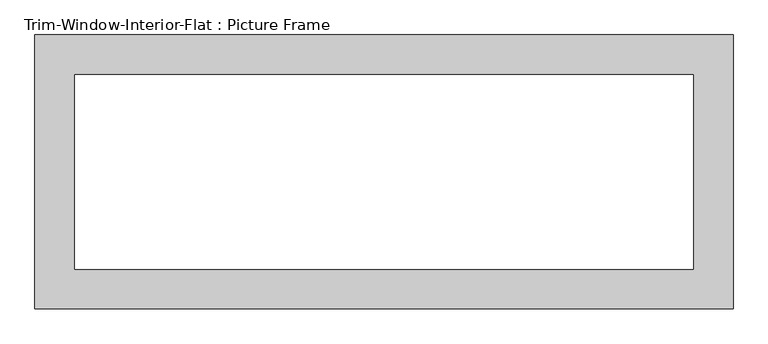
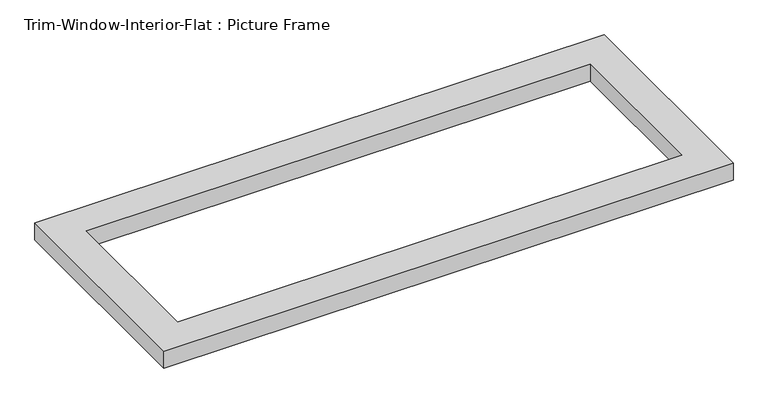
"""IFC4 building model written with IfcOpenShell, lengths in millimetres: proxy geometry, Trim-Window-Interior-Flat : Picture Frame."""

from ifc_helpers import new_model, si_unit, origin, origin_with_axes, place, context, project, spatial, polyline, outline, extrude, source, transform, mapped, element, save


def trim_window_interior_flat_picture_frame_a780e5c2(model_context):
    return source(origin(), model_context, "Body", "SweptSolid", [
        extrude(outline(polyline([(501.65, 44.45), (501.65, -349.25), (-501.65, -349.25), (-501.65, 44.45), (501.65, 44.45)]), holes=[polyline([(444.5, -12.7), (-444.5, -12.7), (-444.5, -292.1), (444.5, -292.1), (444.5, -12.7)])]), origin_with_axes(), (0.0, 0.0, 1.0), 31.75),
    ])


if __name__ == "__main__":
    model = new_model("IFC4")
    model_context = context("Model", 3, world=origin())
    ifc_project = project(units=[si_unit("LENGTHUNIT", "METRE", prefix="MILLI")], contexts=[model_context])
    site = spatial("IfcSite", under=ifc_project)
    building = spatial("IfcBuilding", under=site)
    placement = place(None, origin())
    trim_window_interior_flat_picture_frame_shape = trim_window_interior_flat_picture_frame_a780e5c2(model_context)
    element("IfcBuildingElementProxy", 1, Name="Trim-Window-Interior-Flat : Picture Frame", ObjectType="Trim-Window-Interior-Flat : Picture Frame", at=placement, inside=building, context=model_context, shape_type="MappedRepresentation", body=[
        mapped(trim_window_interior_flat_picture_frame_shape, transform((0.0, 0.0, 0.0), x_axis=(1.0, 0.0, 0.0), y_axis=(0.0, 1.0, 0.0), z_axis=(0.0, 0.0, 1.0))),
    ])
    save(model, "model.ifc")

# Revit data of these elements
# Type "Trim-Window-Interior-Flat : Picture Frame"
#   Trim Thickness_Picture Frame = 0' - 1 1/4"
#   Trim Width = 0' - 2 1/4"
#   Trim Thickness_with Sill = 0' - 0 3/4"
#   Sill Thickness = 0' - 1 1/4"
#   Opening Width [instance default] = 2' - 0"
#   Opening Height [instance default] = 3' - 0"
#   Default Elevation = 4' - 0"
#   Sill = no
#   Picture Frame = yes
#   Trim Material [instance default] = none
# Element 1 (IfcBuildingElementProxy, "Trim-Window-Interior-Flat : Picture Frame")
#   Opening Width = 3' - 0"
#   Opening Height = 1' - 0"
#   Trim Material = Wood - Stained
#   Materials on its faces: "Wood - Stained"
# Materials
#   "Wood - Stained": class "Wood", colour RGB 224 178 126, transparency 0, Cost = 0
